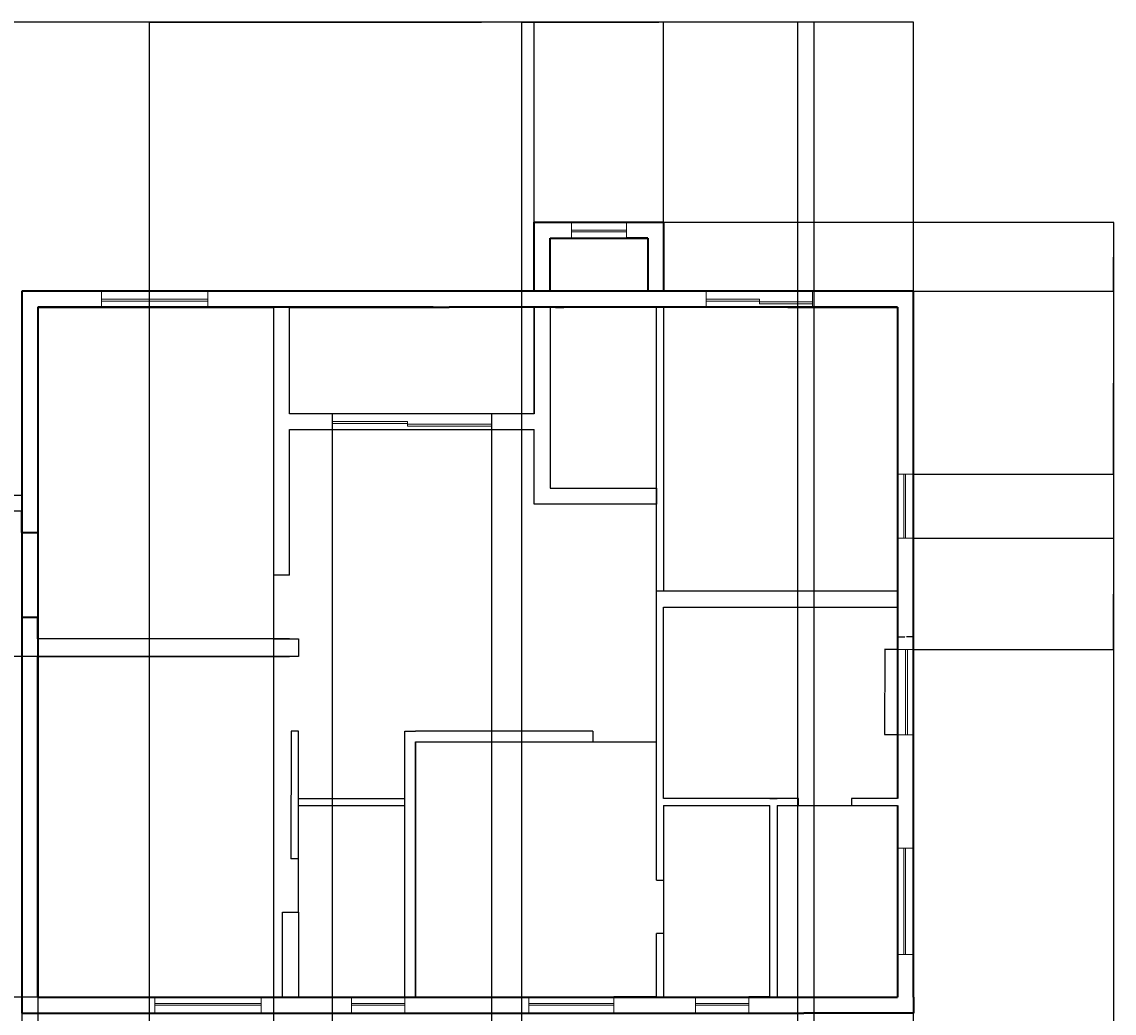
# Model space of a CAD drawing. Units: inches. Extents: x 2029 to 8798, y 1998 to 6373.
# Tile 10 of 11: x 3888 to 4504, y 5814 to 6373. Entities that reach past the tile are written whole.
import ezdxf

# ---------------------------------------------------------------- set-up
doc = ezdxf.new("R2010")
doc.units = ezdxf.units.IN
for name, color, linetype, lineweight in [('A-ANNO-DIMS', 2, 'Continuous', 18), ('A-GLAZ', 4, 'Continuous', 18), ('A-WALL-CIRC', 7, 'Continuous', 25), ('A-WALL-EXTR', 7, 'Continuous', 35), ('A-WALL-INTR', 7, 'Continuous', 25)]:
    doc.layers.add(name, color=color, linetype=linetype, lineweight=lineweight)
doc.styles.get("Standard").update_dxf_attribs({"font": 'arial.ttf'})
doc.dimstyles.get("Standard").update_dxf_attribs({"dimtxt": 0.18, "dimasz": 0.18, "dimexe": 0.18, "dimexo": 0.0625, "dimgap": 0.09, "dimtad": 0, "dimtih": 1, "dimtoh": 1, "dimdec": 4, "dimzin": 0, "dimdsep": 46, "dimtxsty": 'Standard', "dimcen": 0.09, "dimadec": 0, "dimazin": 0, "dimtfac": 1, "dimtdec": 4, "dimtofl": 0, "dimtmove": 0, "dimatfit": 3, "dimfxl": 1, "dimtolj": 1, "dimtzin": 0, "dimarcsym": 0})

# ---------------------------------------------------------------- blocks, each defined once
blk = doc.blocks.new('WIN-60')
for p, q in [((0, 0), (0, 9)), ((60, 9), (60, 0)), ((0, 4.5), (60, 4.5)), ((0, 3.5), (60, 3.5))]:
    blk.add_line(p, q)
blk = doc.blocks.new('WIN-36')
for p, q in [((0, 36), (9, 36)), ((3.5, 36), (3.5, 0)), ((4.5, 36), (4.5, 0)), ((9, 0), (0, 0))]:
    blk.add_line(p, q)
blk = doc.blocks.new('WIN-48')
for p, q in [((0, 48), (9, 48)), ((4.5, 48), (4.5, 0)), ((5.5, 48), (5.5, 0)), ((9, 0), (0, 0))]:
    blk.add_line(p, q)
blk = doc.blocks.new('WIN-30')
for p, q in [((0, 0), (0, 9)), ((30, 9), (30, 0)), ((0, 5.5), (30, 5.5)), ((0, 4.5), (30, 4.5))]:
    blk.add_line(p, q)
blk = doc.blocks.new('*D15')
at = {"layer": 'A-ANNO-DIMS', "color": 0, "lineweight": -2, "transparency": 16777216}
for p, q in [((4381.7, 6018.61), (4374.39, 6018.61)), ((4374.57, 6018.43), (4374.57, 5994.8)), ((4374.57, 5970.79), (4374.57, 5994.43)), ((4381.7, 5970.61), (4374.39, 5970.61))]:
    blk.add_line(p, q, dxfattribs=at)
at = {"layer": 'A-ANNO-DIMS', "color": 0, "transparency": 16777216}
for points in [[(4374.54, 6018.43), (4374.6, 6018.43), (4374.57, 6018.61)], [(4374.54, 5970.79), (4374.6, 5970.79), (4374.57, 5970.61)]]:
    blk.add_solid(points, dxfattribs=at)
at = {"layer": 'Defpoints', "color": 0, "transparency": 16777216}
for p in [(4374.57, 6018.61), (4381.77, 6018.61), (4381.77, 5970.61)]:
    blk.add_point(p, dxfattribs=at)
at = {"layer": 'A-ANNO-DIMS', "color": 0, "transparency": 16777216, "insert": (4374.57, 5994.61), "char_height": 0.18, "attachment_point": 5}
blk.add_mtext('\\A1;WINDOW 48 TYP.', dxfattribs=at)
blk = doc.blocks.new('*D16')
at = {"layer": 'A-ANNO-DIMS', "color": 0, "lineweight": -2, "transparency": 16777216}
for p, q in [((4381.77, 6018.67), (4381.77, 6025.99)), ((4381.95, 6025.81), (4385.81, 6025.81)), ((4390.59, 6025.81), (4386.72, 6025.81)), ((4390.77, 6018.67), (4390.77, 6025.99))]:
    blk.add_line(p, q, dxfattribs=at)
at = {"layer": 'A-ANNO-DIMS', "color": 0, "transparency": 16777216}
for points in [[(4381.95, 6025.84), (4381.95, 6025.78), (4381.77, 6025.81)], [(4390.59, 6025.84), (4390.59, 6025.78), (4390.77, 6025.81)]]:
    blk.add_solid(points, dxfattribs=at)
at = {"layer": 'Defpoints', "color": 0, "transparency": 16777216}
for p in [(4390.77, 6025.81), (4381.77, 6018.61), (4390.77, 6018.61)]:
    blk.add_point(p, dxfattribs=at)
at = {"layer": 'A-ANNO-DIMS', "color": 0, "transparency": 16777216, "insert": (4386.27, 6025.81), "char_height": 0.18, "attachment_point": 5}
blk.add_mtext('\\A1;9 TYP.', dxfattribs=at)
blk = doc.blocks.new('*D77')
at = {"layer": 'A-ANNO-DIMS', "color": 0, "lineweight": -2, "transparency": 16777216}
for p, q in [((3959.77, 5121.16), (3959.77, 6372.54)), ((3959.95, 6372.36), (4146.98, 6372.36)), ((4334.59, 6372.36), (4147.56, 6372.36)), ((4334.77, 5121.16), (4334.77, 6372.54))]:
    blk.add_line(p, q, dxfattribs=at)
at = {"layer": 'A-ANNO-DIMS', "color": 0, "transparency": 16777216}
for points in [[(3959.95, 6372.39), (3959.95, 6372.33), (3959.77, 6372.36)], [(4334.59, 6372.39), (4334.59, 6372.33), (4334.77, 6372.36)]]:
    blk.add_solid(points, dxfattribs=at)
at = {"layer": 'Defpoints', "color": 0, "transparency": 16777216}
for p in [(4334.77, 6372.36), (3959.77, 5121.09), (4334.77, 5121.09)]:
    blk.add_point(p, dxfattribs=at)
at = {"layer": 'A-ANNO-DIMS', "color": 0, "transparency": 16777216, "insert": (4147.27, 6372.36), "char_height": 0.18, "attachment_point": 5}
blk.add_mtext('\\A1;375', dxfattribs=at)
blk = doc.blocks.new('*D78')
at = {"layer": 'A-ANNO-DIMS', "color": 0, "lineweight": -2, "transparency": 16777216}
for p, q in [((3896.77, 6211.55), (3896.77, 4031.06)), ((4029.77, 6211.55), (4029.77, 4031.06)), ((3896.95, 4031.24), (3962.99, 4031.24)), ((4029.59, 4031.24), (3963.55, 4031.24))]:
    blk.add_line(p, q, dxfattribs=at)
at = {"layer": 'A-ANNO-DIMS', "color": 0, "transparency": 16777216}
for points in [[(3896.95, 4031.27), (3896.95, 4031.21), (3896.77, 4031.24)], [(4029.59, 4031.27), (4029.59, 4031.21), (4029.77, 4031.24)]]:
    blk.add_solid(points, dxfattribs=at)
at = {"layer": 'Defpoints', "color": 0, "transparency": 16777216}
for p in [(3896.77, 6211.61), (4029.77, 6211.61), (4029.77, 4031.24)]:
    blk.add_point(p, dxfattribs=at)
at = {"layer": 'A-ANNO-DIMS', "color": 0, "transparency": 16777216, "insert": (3963.27, 4031.24), "char_height": 0.18, "attachment_point": 5}
blk.add_mtext('\\A1;133', dxfattribs=at)
blk = doc.blocks.new('*D79')
at = {"layer": 'A-ANNO-DIMS', "color": 0, "lineweight": -2, "transparency": 16777216}
for p, q in [((4043.7, 6014.61), (2029.61, 6014.61)), ((2029.79, 6014.43), (2029.79, 5918.79)), ((2029.79, 5822.79), (2029.79, 5918.43)), ((4043.7, 5822.61), (2029.61, 5822.61))]:
    blk.add_line(p, q, dxfattribs=at)
at = {"layer": 'A-ANNO-DIMS', "color": 0, "transparency": 16777216}
for points in [[(2029.76, 6014.43), (2029.82, 6014.43), (2029.79, 6014.61)], [(2029.76, 5822.79), (2029.82, 5822.79), (2029.79, 5822.61)]]:
    blk.add_solid(points, dxfattribs=at)
at = {"layer": 'Defpoints', "color": 0, "transparency": 16777216}
for p in [(2029.79, 6014.61), (4043.77, 6014.61), (4043.77, 5822.61)]:
    blk.add_point(p, dxfattribs=at)
at = {"layer": 'A-ANNO-DIMS', "color": 0, "transparency": 16777216, "insert": (2029.79, 5918.61), "char_height": 0.18, "attachment_point": 5}
blk.add_mtext('\\A1;192', dxfattribs=at)
blk = doc.blocks.new('*D80')
at = {"layer": 'A-ANNO-DIMS', "color": 0, "lineweight": -2, "transparency": 16777216}
for p, q in [((4390.83, 6220.61), (4503.7, 6220.61)), ((4503.52, 6220.43), (4503.52, 6169.24)), ((4503.52, 6117.68), (4503.52, 6168.87)), ((4390.83, 6117.5), (4503.7, 6117.5))]:
    blk.add_line(p, q, dxfattribs=at)
at = {"layer": 'A-ANNO-DIMS', "color": 0, "transparency": 16777216}
for points in [[(4503.49, 6220.43), (4503.55, 6220.43), (4503.52, 6220.61)], [(4503.49, 6117.68), (4503.55, 6117.68), (4503.52, 6117.5)]]:
    blk.add_solid(points, dxfattribs=at)
at = {"layer": 'Defpoints', "color": 0, "transparency": 16777216}
for p in [(4390.77, 6220.61), (4390.77, 6117.5), (4503.52, 6117.5)]:
    blk.add_point(p, dxfattribs=at)
at = {"layer": 'A-ANNO-DIMS', "color": 0, "transparency": 16777216, "insert": (4503.52, 6169.05), "char_height": 0.18, "attachment_point": 5}
blk.add_mtext('\\A1;103.12', dxfattribs=at)
blk = doc.blocks.new('*D81')
at = {"layer": 'A-ANNO-DIMS', "color": 0, "lineweight": -2, "transparency": 16777216}
for p, q in [((4390.83, 6081.5), (4503.7, 6081.5)), ((4503.52, 6081.32), (4503.52, 6050.24)), ((4503.52, 6018.79), (4503.52, 6049.87)), ((4390.83, 6018.61), (4503.7, 6018.61))]:
    blk.add_line(p, q, dxfattribs=at)
at = {"layer": 'A-ANNO-DIMS', "color": 0, "transparency": 16777216}
for points in [[(4503.49, 6081.32), (4503.55, 6081.32), (4503.52, 6081.5)], [(4503.49, 6018.79), (4503.55, 6018.79), (4503.52, 6018.61)]]:
    blk.add_solid(points, dxfattribs=at)
at = {"layer": 'Defpoints', "color": 0, "transparency": 16777216}
for p in [(4390.77, 6081.5), (4390.77, 6018.61), (4503.52, 6018.61)]:
    blk.add_point(p, dxfattribs=at)
at = {"layer": 'A-ANNO-DIMS', "color": 0, "transparency": 16777216, "insert": (4503.52, 6050.05), "char_height": 0.18, "attachment_point": 5}
blk.add_mtext('\\A1;62.88', dxfattribs=at)
blk = doc.blocks.new('*D82')
at = {"layer": 'A-ANNO-DIMS', "color": 0, "lineweight": -2, "transparency": 16777216}
for p, q in [((4249.83, 6259.61), (4503.7, 6259.61)), ((4503.52, 6259.43), (4503.52, 6240.29)), ((4503.52, 6220.79), (4503.52, 6239.93)), ((4249.83, 6220.61), (4503.7, 6220.61))]:
    blk.add_line(p, q, dxfattribs=at)
at = {"layer": 'A-ANNO-DIMS', "color": 0, "transparency": 16777216}
for points in [[(4503.49, 6259.43), (4503.55, 6259.43), (4503.52, 6259.61)], [(4503.49, 6220.79), (4503.55, 6220.79), (4503.52, 6220.61)]]:
    blk.add_solid(points, dxfattribs=at)
at = {"layer": 'Defpoints', "color": 0, "transparency": 16777216}
for p in [(4249.77, 6259.61), (4249.77, 6220.61), (4503.52, 6220.61)]:
    blk.add_point(p, dxfattribs=at)
at = {"layer": 'A-ANNO-DIMS', "color": 0, "transparency": 16777216, "insert": (4503.52, 6240.11), "char_height": 0.18, "attachment_point": 5}
blk.add_mtext('\\A1;39', dxfattribs=at)
blk = doc.blocks.new('*D83')
at = {"layer": 'A-ANNO-DIMS', "color": 0, "lineweight": -2, "transparency": 16777216}
for p, q in [((4062.77, 6151.55), (4062.77, 4031.06)), ((4152.77, 6151.55), (4152.77, 4031.06)), ((4062.95, 4031.24), (4107.55, 4031.24)), ((4152.59, 4031.24), (4107.98, 4031.24))]:
    blk.add_line(p, q, dxfattribs=at)
at = {"layer": 'A-ANNO-DIMS', "color": 0, "transparency": 16777216}
for points in [[(4062.95, 4031.27), (4062.95, 4031.21), (4062.77, 4031.24)], [(4152.59, 4031.27), (4152.59, 4031.21), (4152.77, 4031.24)]]:
    blk.add_solid(points, dxfattribs=at)
at = {"layer": 'Defpoints', "color": 0, "transparency": 16777216}
for p in [(4062.77, 6151.61), (4152.77, 6151.61), (4152.77, 4031.24)]:
    blk.add_point(p, dxfattribs=at)
at = {"layer": 'A-ANNO-DIMS', "color": 0, "transparency": 16777216, "insert": (4107.77, 4031.24), "char_height": 0.18, "attachment_point": 5}
blk.add_mtext('\\A1;90', dxfattribs=at)
blk = doc.blocks.new('*D88')
at = {"layer": 'A-ANNO-DIMS', "color": 0, "lineweight": -2, "transparency": 16777216}
for p, q in [((2142.54, 4445.05), (2142.54, 6372.54)), ((2142.72, 6372.36), (3266.19, 6372.36)), ((4390.59, 6372.36), (3267.12, 6372.36)), ((4390.77, 4574.05), (4390.77, 6372.54))]:
    blk.add_line(p, q, dxfattribs=at)
at = {"layer": 'A-ANNO-DIMS', "color": 0, "transparency": 16777216}
for points in [[(2142.72, 6372.39), (2142.72, 6372.33), (2142.54, 6372.36)], [(4390.59, 6372.39), (4390.59, 6372.33), (4390.77, 6372.36)]]:
    blk.add_solid(points, dxfattribs=at)
at = {"layer": 'Defpoints', "color": 0, "transparency": 16777216}
for p in [(4390.77, 6372.36), (4390.77, 4573.99), (2142.54, 4444.99)]:
    blk.add_point(p, dxfattribs=at)
at = {"layer": 'A-ANNO-DIMS', "color": 0, "transparency": 16777216, "insert": (3266.65, 6372.36), "char_height": 0.18, "attachment_point": 5}
blk.add_mtext('\\A1;2248.2', dxfattribs=at)
blk = doc.blocks.new('*D89')
at = {"layer": 'A-ANNO-DIMS', "color": 0, "lineweight": -2, "transparency": 16777216}
for p, q in [((4249.83, 6259.61), (4503.7, 6259.61)), ((4503.52, 6259.43), (4503.52, 5201.98)), ((4503.52, 4144.17), (4503.52, 5201.62)), ((4105.83, 4143.99), (4503.7, 4143.99))]:
    blk.add_line(p, q, dxfattribs=at)
at = {"layer": 'A-ANNO-DIMS', "color": 0, "transparency": 16777216}
for points in [[(4503.49, 6259.43), (4503.55, 6259.43), (4503.52, 6259.61)], [(4503.49, 4144.17), (4503.55, 4144.17), (4503.52, 4143.99)]]:
    blk.add_solid(points, dxfattribs=at)
at = {"layer": 'Defpoints', "color": 0, "transparency": 16777216}
for p in [(4249.77, 6259.61), (4503.52, 6259.61), (4105.77, 4143.99)]:
    blk.add_point(p, dxfattribs=at)
at = {"layer": 'A-ANNO-DIMS', "color": 0, "transparency": 16777216, "insert": (4503.52, 5201.8), "char_height": 0.18, "attachment_point": 5}
blk.add_mtext('\\A1;2115.6', dxfattribs=at)
blk = doc.blocks.new('*D109')
at = {"layer": 'A-ANNO-DIMS', "color": 0, "lineweight": -2, "transparency": 16777216}
for p, q in [((4169.77, 4992.16), (4169.77, 6372.54)), ((4169.95, 6372.36), (4247.12, 6372.36)), ((4325.21, 6372.36), (4248.03, 6372.36)), ((4325.39, 4992.16), (4325.39, 6372.54))]:
    blk.add_line(p, q, dxfattribs=at)
at = {"layer": 'A-ANNO-DIMS', "color": 0, "transparency": 16777216}
for points in [[(4169.95, 6372.39), (4169.95, 6372.33), (4169.77, 6372.36)], [(4325.21, 6372.39), (4325.21, 6372.33), (4325.39, 6372.36)]]:
    blk.add_solid(points, dxfattribs=at)
at = {"layer": 'Defpoints', "color": 0, "transparency": 16777216}
for p in [(4325.39, 6372.36), (4169.77, 4992.09), (4325.39, 4992.09)]:
    blk.add_point(p, dxfattribs=at)
at = {"layer": 'A-ANNO-DIMS', "color": 0, "transparency": 16777216, "insert": (4247.58, 6372.36), "char_height": 0.18, "attachment_point": 5}
blk.add_mtext('\\A1;155.62', dxfattribs=at)
blk = doc.blocks.new('*D118')
at = {"layer": 'A-ANNO-DIMS', "color": 0, "lineweight": -2, "transparency": 16777216}
for p, q in [((4176.77, 6259.67), (4176.77, 6372.54)), ((4176.95, 6372.36), (4213.05, 6372.36)), ((4249.59, 6372.36), (4213.48, 6372.36)), ((4249.77, 6259.67), (4249.77, 6372.54))]:
    blk.add_line(p, q, dxfattribs=at)
at = {"layer": 'A-ANNO-DIMS', "color": 0, "transparency": 16777216}
for points in [[(4176.95, 6372.39), (4176.95, 6372.33), (4176.77, 6372.36)], [(4249.59, 6372.39), (4249.59, 6372.33), (4249.77, 6372.36)]]:
    blk.add_solid(points, dxfattribs=at)
at = {"layer": 'Defpoints', "color": 0, "transparency": 16777216}
for p in [(4249.77, 6372.36), (4176.77, 6259.61), (4249.77, 6259.61)]:
    blk.add_point(p, dxfattribs=at)
at = {"layer": 'A-ANNO-DIMS', "color": 0, "transparency": 16777216, "insert": (4213.27, 6372.36), "char_height": 0.18, "attachment_point": 5}
blk.add_mtext('\\A1;73', dxfattribs=at)

msp = doc.modelspace()

# ---------------------------------------------------------------- linework, layer by layer
at = {"layer": 'A-GLAZ'}
for p, q in [((4197.7657, 6250.6123), (4197.7657, 6259.6123)), ((4197.7657, 6255.1123), (4228.7657, 6255.1123)), ((4197.7657, 6254.1123), (4228.7657, 6254.1123)), ((4228.7657, 6250.6123), (4228.7657, 6259.6123)), ((4273.7657, 6211.6123), (4273.7657, 6220.6123)), ((4273.7657, 6220.6123), (4333.7657, 6220.6123)), ((4333.7657, 6220.6123), (4333.7657, 6211.6123)), ((4273.7657, 6216.1123), (4303.9284, 6216.1123)), ((4303.9284, 6215.1123), (4273.7657, 6215.1123)), ((4303.9284, 6216.1123), (4303.9284, 6215.1123)), ((4303.9284, 6214.6123), (4333.7657, 6214.6123)), ((4303.9284, 6213.6123), (4303.9284, 6214.6123)), ((4333.7657, 6213.6123), (4303.9284, 6213.6123)), ((4333.7657, 6214.6123), (4333.7657, 6213.6123)), ((4062.7657, 6142.6123), (4062.7657, 6151.6123)), ((4152.7657, 6142.6123), (4152.7657, 6151.6123)), ((4062.7657, 6147.1123), (4105.3183, 6147.1123)), ((4105.3183, 6146.1123), (4062.7657, 6146.1123)), ((4105.3183, 6147.1123), (4105.3183, 6146.1123)), ((4105.3183, 6145.6123), (4152.7657, 6145.6123)), ((4105.3183, 6144.6123), (4105.3183, 6145.6123)), ((4152.7657, 6144.6123), (4105.3183, 6144.6123)), ((4152.7657, 6145.6123), (4152.7657, 6144.6123)), ((4390.7657, 6117.4966), (4390.7657, 6081.4966)), ((4390.7657, 6018.6123), (4390.7657, 5970.6123)), ((4103.7657, 5813.6123), (4073.7657, 5813.6123)), ((4221.7657, 5813.6123), (4173.7657, 5813.6123))]:
    msp.add_line(p, q, dxfattribs=at)
at = {"layer": 'A-WALL-CIRC'}
for p, q in [((3809.7657, 6105.6123), (3887.7657, 6105.6123)), ((3887.7657, 6096.6123), (3809.7657, 6096.6123)), ((3896.7657, 5822.6123), (3896.7657, 5672.6123)), ((3887.7657, 5813.6123), (3887.7657, 5663.6123))]:
    msp.add_line(p, q, dxfattribs=at)
at = {"layer": 'A-WALL-EXTR'}
for p, q in [((4176.7657, 6220.6123), (4176.7657, 6259.6123)), ((4176.7657, 6259.6123), (4249.7657, 6259.6123)), ((4249.7657, 6259.6123), (4249.7657, 6220.6123)), ((4185.7657, 6220.6123), (4185.7657, 6250.6123)), ((4185.7657, 6250.6123), (4240.7657, 6250.6123)), ((4185.7657, 6250.6123), (4197.7657, 6250.6123)), ((4240.7657, 6250.6123), (4228.7657, 6250.6123)), ((4240.7657, 6250.6123), (4240.7657, 6220.6123)), ((3968.7657, 6220.6123), (3887.7657, 6220.6123)), ((3887.7657, 6220.6123), (3887.7657, 5813.6123)), ((4110.7657, 6220.6123), (3968.7657, 6220.6123)), ((4328.7657, 6220.6123), (4110.7657, 6220.6123)), ((4390.7657, 6220.6123), (4328.7657, 6220.6123)), ((4390.7657, 5822.6123), (4390.7657, 6220.6123)), ((3968.7657, 6211.6123), (3896.7657, 6211.6123)), ((3896.7657, 6211.6123), (3896.7657, 5822.6123)), ((3896.7657, 6211.6123), (4029.7657, 6211.6123)), ((3896.7657, 6211.6123), (3896.7657, 6211.6123)), ((4110.7657, 6211.6123), (3968.7657, 6211.6123)), ((4038.7657, 6211.6123), (4119.7657, 6211.6123)), ((4119.7657, 6211.6123), (4110.7657, 6211.6123)), ((4119.7657, 6211.6123), (4128.7657, 6211.6123)), ((4188.7657, 6211.6123), (4128.7657, 6211.6123)), ((4245.7657, 6211.6123), (4185.7657, 6211.6123)), ((4188.7657, 6211.6123), (4193.417, 6211.6123)), ((4319.7657, 6211.6123), (4192.7657, 6211.6123)), ((4381.7657, 6211.6123), (4249.7657, 6211.6123)), ((4319.7657, 6211.6123), (4381.7657, 6211.6123)), ((4381.7657, 6211.6123), (4381.7657, 5934.6123)), ((4381.7657, 6211.6123), (4381.7657, 6051.6123)), ((4381.7657, 6211.6123), (4381.7657, 6117.4966)), ((3887.7657, 6084.6123), (3887.7657, 6096.6123)), ((3887.7657, 6084.6123), (3896.7657, 6084.6123)), ((4381.7657, 6042.6123), (4381.7657, 5934.6123)), ((3896.7657, 6036.6123), (3887.7657, 6036.6123)), ((3896.7657, 6024.6123), (3896.7657, 6036.6123)), ((3896.7657, 5822.6123), (3896.7657, 6014.6123)), ((4381.7657, 5930.6123), (4381.7657, 5822.6123)), ((3896.7657, 5822.6123), (4034.7657, 5822.6123)), ((4034.7657, 5822.6123), (4107.7657, 5822.6123)), ((4107.7657, 5822.6123), (4251.7657, 5822.6123)), ((4245.7657, 5822.6123), (4221.7657, 5822.6123)), ((4251.7657, 5822.6123), (4319.7657, 5822.6123)), ((4309.7657, 5822.6123), (4297.7657, 5822.6123)), ((4313.7657, 5822.6123), (4381.7657, 5822.6123)), ((4390.7657, 5822.6123), (4390.7657, 5813.6123)), ((3887.7657, 5813.6123), (4034.7657, 5813.6123)), ((4034.7657, 5813.6123), (4107.7657, 5813.6123)), ((4107.7657, 5813.6123), (4251.7657, 5813.6123)), ((4251.7657, 5813.6123), (4328.7657, 5813.6123)), ((4390.7657, 5813.6123), (4328.7657, 5813.6123))]:
    msp.add_line(p, q, dxfattribs=at)
at = {"layer": 'A-WALL-INTR'}
for p, q in [((4029.7657, 6211.6123), (4029.7657, 6024.6123)), ((4038.7657, 6151.6123), (4038.7657, 6211.6123)), ((4176.7657, 6211.6123), (4176.7657, 6151.6123)), ((4176.7657, 6151.6123), (4176.7657, 6211.6123)), ((4185.7657, 6211.6123), (4185.7657, 6109.6123)), ((4245.7657, 6051.6123), (4245.7657, 6211.6123)), ((4249.7657, 6211.6123), (4249.7657, 6051.6123)), ((4176.7657, 6151.6123), (4038.7657, 6151.6123)), ((4038.7657, 6060.6123), (4038.7657, 6142.6123)), ((4038.7657, 6142.6123), (4176.7657, 6142.6123)), ((4176.7657, 6100.6123), (4176.7657, 6142.6123)), ((4185.7657, 6109.6123), (4245.7657, 6109.6123)), ((4245.7657, 6109.6123), (4245.7657, 6100.6123)), ((4245.7657, 6100.6123), (4176.7657, 6100.6123)), ((4038.7657, 6060.6123), (4029.7657, 6060.6123)), ((4381.7657, 6051.6123), (4245.7657, 6051.6123)), ((4245.7657, 6042.6123), (4245.7657, 6051.6123)), ((4249.7657, 6051.6123), (4245.7657, 6051.6123)), ((4245.7657, 5930.6123), (4245.7657, 6042.6123)), ((4249.7657, 6042.6123), (4381.7657, 6042.6123)), ((4249.7657, 5934.6123), (4249.7657, 6042.6123)), ((4038.7657, 6024.6123), (3896.7657, 6024.6123)), ((4029.7657, 6024.6123), (4038.7657, 6024.6123)), ((4038.7657, 6024.6123), (4043.7657, 6024.6123)), ((4043.7657, 6024.6123), (4043.7657, 6014.6123)), ((3896.7657, 6014.6123), (4038.7657, 6014.6123)), ((4043.7657, 6014.6123), (4038.7657, 6014.6123)), ((4039.7657, 5972.6123), (4039.4129, 5900.6336)), ((4043.7657, 5972.6123), (4039.7657, 5972.6123)), ((4043.7657, 5870.6123), (4043.7657, 5972.6123)), ((4103.7657, 5822.6123), (4103.7657, 5972.6123)), ((4103.7657, 5972.6123), (4109.7657, 5972.6123)), ((4209.7657, 5972.6123), (4109.7657, 5972.6123)), ((4209.7657, 5972.6123), (4209.7657, 5966.6123)), ((4245.7657, 5966.6123), (4245.7657, 5972.6123)), ((4109.7657, 5966.6123), (4109.7657, 5822.6123)), ((4109.7657, 5822.6123), (4109.7657, 5966.6123)), ((4109.7657, 5966.6123), (4245.7657, 5966.6123)), ((4043.7657, 5934.6123), (4103.7657, 5934.6123)), ((4325.7657, 5934.6123), (4249.7657, 5934.6123)), ((4309.7657, 5934.6123), (4313.7657, 5934.6123)), ((4325.7657, 5930.6123), (4325.7657, 5934.6123)), ((4381.7657, 5934.6123), (4355.7657, 5934.6123)), ((4355.7657, 5934.6123), (4355.7657, 5930.6123)), ((4043.7657, 5930.6123), (4103.7657, 5930.6123)), ((4245.7657, 5888.6123), (4245.7657, 5930.6123)), ((4249.7657, 5930.6123), (4249.7657, 5822.6123)), ((4249.7657, 5930.6123), (4309.7657, 5930.6123)), ((4309.7657, 5822.6123), (4309.7657, 5930.6123)), ((4313.7657, 5930.6123), (4313.7657, 5822.6123)), ((4313.7657, 5930.6123), (4381.7657, 5930.6123)), ((4043.7657, 5900.6123), (4039.4129, 5900.6336)), ((4043.7657, 5870.6123), (4043.7657, 5900.6123)), ((4043.7657, 5870.6123), (4043.7657, 5900.6123)), ((4245.7657, 5888.6123), (4249.7657, 5888.6123)), ((4034.7657, 5822.6123), (4034.7657, 5870.6123)), ((4034.7657, 5870.6123), (4043.7657, 5870.6123)), ((4043.7657, 5870.6123), (4043.7657, 5822.6123)), ((4245.7657, 5822.6123), (4245.7657, 5858.6123)), ((4249.7657, 5858.6123), (4245.7657, 5858.6123))]:
    msp.add_line(p, q, dxfattribs=at)

# ---------------------------------------------------------------- block references
at = {"layer": 'A-GLAZ'}
for name, p in [('WIN-60', (3932.7657, 6211.6123)), ('WIN-36', (4381.7657, 6081.4966)), ('WIN-48', (4381.7657, 5970.6123)), ('WIN-30', (4073.7657, 5813.6123)), ('WIN-30', (4267.7657, 5813.6123))]:
    msp.add_blockref(name, p, dxfattribs=at)
at = {"layer": 'A-GLAZ', "extrusion": (0, 0, -1), "zscale": -1}
for name, p, rotation in [('WIN-60', (-4381.7657, 5846.6123), 90), ('WIN-60', (-3962.7657, 5822.6123), 180), ('WIN-48', (-4173.7657, 5813.6123), 90)]:
    msp.add_blockref(name, p, dxfattribs=dict(at, rotation=rotation))

# ---------------------------------------------------------------- dimensions: what is measured, and where the dimension line sits
at = {"layer": 'A-ANNO-DIMS'}
for base, p1, p2, override, picture, middle in [((4390.7657, 6372.3623), (2142.5398, 4444.9886), (4390.7657, 4573.9886), {"dimdec": 1, "dimlfac": 1, "dimrnd": 0, "dimzin": 0, "dimdsep": 46, "dimlunit": 2}, '*D88', (3266.6528, 6372.3623)), ((4334.7657, 6372.3623), (3959.7657, 5121.0948), (4334.7657, 5121.0948), {"dimdec": 0, "dimlfac": 1, "dimrnd": 0, "dimzin": 0, "dimdsep": 46, "dimlunit": 2}, '*D77', (4147.2657, 6372.3623)), ((4325.3869, 6372.3623), (4169.7657, 4992.0948), (4325.3869, 4992.0948), {"dimdec": 2, "dimlfac": 1, "dimrnd": 0, "dimzin": 0, "dimdsep": 46, "dimlunit": 2}, '*D109', (4247.5763, 6372.3623)), ((4249.7657, 6372.3623), (4176.7657, 6259.6123), (4249.7657, 6259.6123), {"dimdec": 0, "dimlfac": 1, "dimrnd": 0, "dimzin": 0, "dimdsep": 46, "dimlunit": 2}, '*D118', (4213.2657, 6372.3623)), ((4029.7657, 4031.2386), (3896.7657, 6211.6123), (4029.7657, 6211.6123), {"dimdec": 0, "dimlfac": 1, "dimrnd": 0, "dimzin": 0, "dimdsep": 46, "dimlunit": 2}, '*D78', (3963.2657, 4031.2386)), ((4152.7657, 4031.2386), (4062.7657, 6151.6123), (4152.7657, 6151.6123), {"dimdec": 0, "dimlfac": 1, "dimrnd": 0, "dimzin": 0, "dimdsep": 46, "dimlunit": 2}, '*D83', (4107.7657, 4031.2386))]:
    dim = msp.add_linear_dim(base=base, p1=p1, p2=p2, dimstyle='Standard', override=override, dxfattribs=at)
    dim.commit()
    dim.dimension.update_dxf_attribs({"geometry": picture, "text_midpoint": middle})
for base, p1, p2, override, picture, middle in [((4503.5157, 6259.6123), (4105.7657, 4143.9886), (4249.7657, 6259.6123), {"dimdec": 1, "dimlfac": 1, "dimrnd": 0, "dimzin": 0, "dimdsep": 46, "dimlunit": 2}, '*D89', (4503.5157, 5201.8004)), ((4503.5157, 6220.6123), (4249.7657, 6259.6123), (4249.7657, 6220.6123), {"dimdec": 0, "dimlfac": 1, "dimrnd": 0, "dimzin": 0, "dimdsep": 46, "dimlunit": 2}, '*D82', (4503.5157, 6240.1123)), ((4503.5157, 6117.4966), (4390.7657, 6220.6123), (4390.7657, 6117.4966), {"dimdec": 2, "dimlfac": 1, "dimrnd": 0, "dimzin": 0, "dimdsep": 46, "dimlunit": 2}, '*D80', (4503.5157, 6169.0545)), ((4503.5157, 6018.6123), (4390.7657, 6081.4966), (4390.7657, 6018.6123), {"dimdec": 2, "dimlfac": 1, "dimrnd": 0, "dimzin": 0, "dimdsep": 46, "dimlunit": 2}, '*D81', (4503.5157, 6050.0545)), ((2029.7898, 6014.6123), (4043.7657, 5822.6123), (4043.7657, 6014.6123), {"dimdec": 0, "dimlfac": 1, "dimrnd": 0, "dimzin": 0, "dimdsep": 46, "dimlunit": 2}, '*D79', (2029.7898, 5918.6123))]:
    dim = msp.add_linear_dim(base=base, p1=p1, p2=p2, angle=90, dimstyle='Standard', override=override, dxfattribs=at)
    dim.commit()
    dim.dimension.update_dxf_attribs({"geometry": picture, "text_midpoint": middle})
dim = msp.add_linear_dim(base=(4390.7657, 6025.8123), p1=(4381.7657, 6018.6123), p2=(4390.7657, 6018.6123), text='<> TYP.', dimstyle='Standard', override={"dimdec": 0, "dimlfac": 1, "dimrnd": 0, "dimzin": 0, "dimdsep": 46, "dimlunit": 2}, dxfattribs=at)
dim.commit()
dim.dimension.update_dxf_attribs({"geometry": '*D16', "text_midpoint": (4386.2657, 6025.8123)})
dim = msp.add_linear_dim(base=(4374.5657, 6018.6123), p1=(4381.7657, 5970.6123), p2=(4381.7657, 6018.6123), angle=90, text='WINDOW <> TYP.', dimstyle='Standard', override={"dimdec": 0, "dimlfac": 1, "dimrnd": 0, "dimzin": 0, "dimdsep": 46, "dimlunit": 2}, dxfattribs=at)
dim.commit()
dim.dimension.update_dxf_attribs({"geometry": '*D15', "text_midpoint": (4374.5657, 5994.6123)})

doc.saveas('drawing.dxf')
